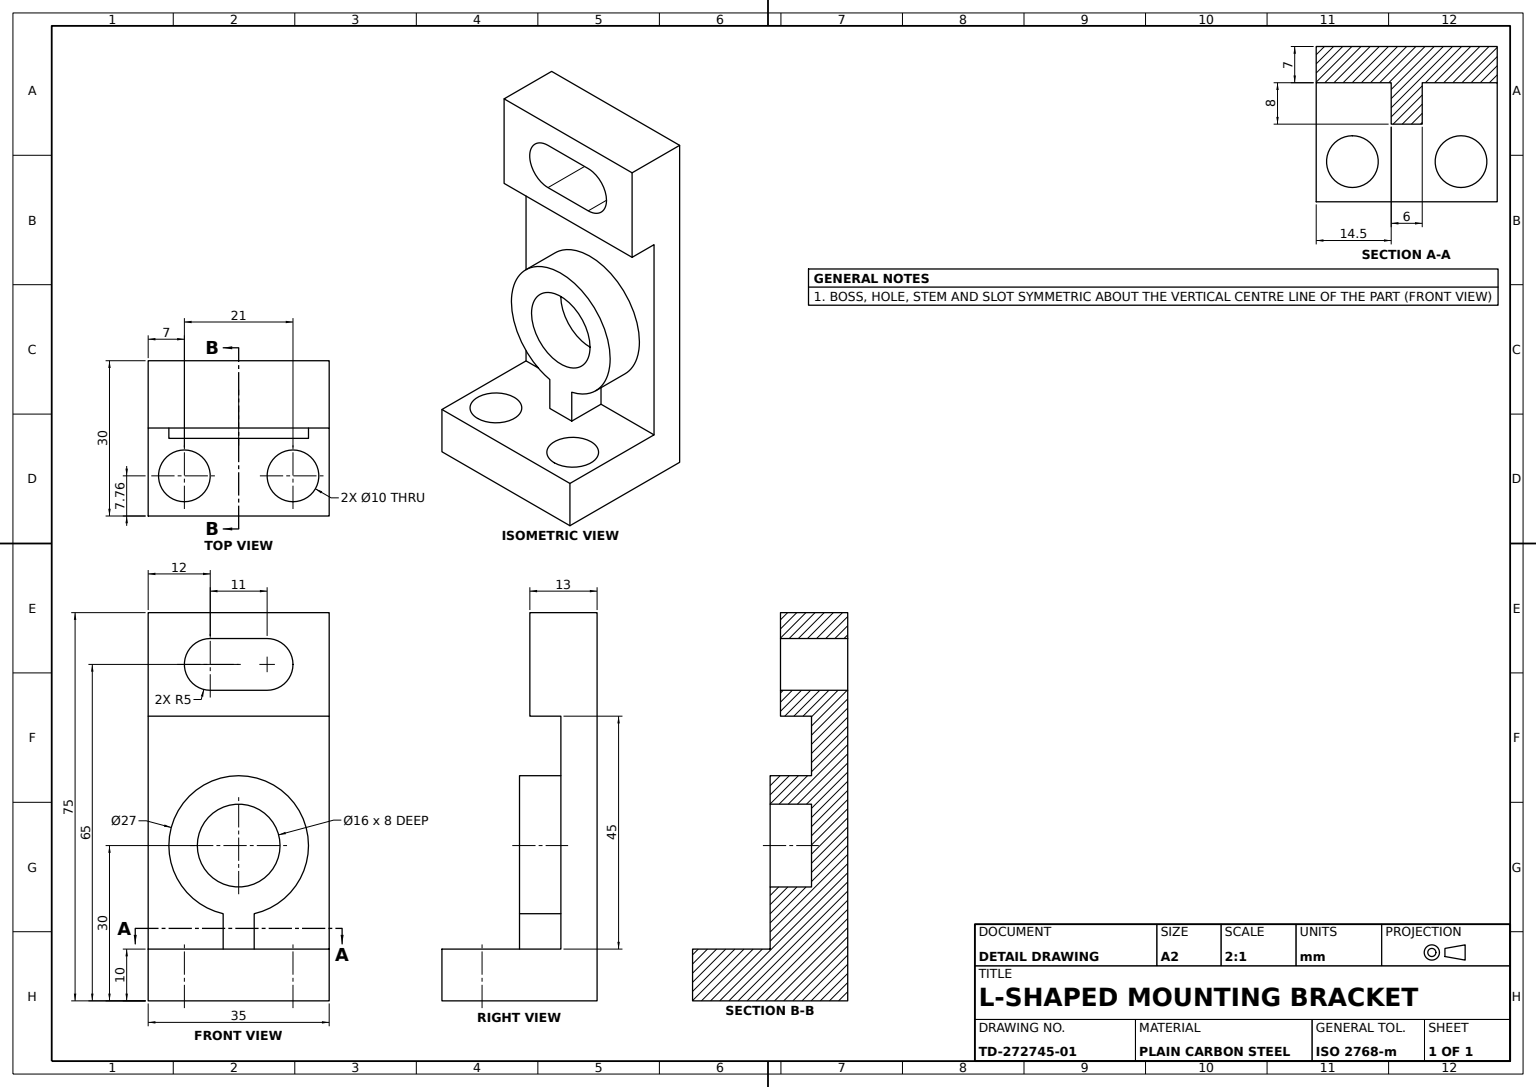
SolidWorks part; units mm, degrees
material "Plain Carbon Steel"
ref_plane "Front Plane" through (0, 0, 0) normal (0, 0, 1) x (1, 0, 0)
ref_plane "Top Plane" through (0, 0, 0) normal (0, 1, 0) x (1, 0, 0)
ref_plane "Right Plane" through (0, 0, 0) normal (1, 0, 0) x (0, 0, -1)
sketch "L-Bracket Profile Sketch" plane through (0, 0, 0) normal (1, 0, 0) x (0, 0, -1)
  line L0 (0, 0) -> (30, 0)
  line L1 (30, 0) -> (30, 10)
  line L2 (30, 10) -> (7, 10)
  line L3 (7, 10) -> (7, 55)
  line L4 (7, 55) -> (13, 55)
  line L5 (13, 55) -> (13, 75)
  line L6 (13, 75) -> (0, 75)
  line L7 (0, 75) -> (0, 0)
  dimension "D1" = 30
  dimension "D2" = 75
  dimension "D3" = 20
  dimension "D4" = 45
  dimension "D5" = 13
  dimension "D6" = 6
extrude "L-Bracket Body" add sketch "L-Bracket Profile Sketch" along normal mid plane 35
sketch "Upright Slot Sketch" plane through (0, 0, -13) normal (0, 0, -1) x (-1, 0, 0)
  line L0 (-5.5, 65) -> (5.5, 65) construction
  line L1 (-5.5, 70) -> (5.5, 70)
  line L2 (-5.5, 60) -> (5.5, 60)
  arc A0 (-5.5, 70) -> (-5.5, 60) centre (-5.5, 65) ccw
  arc A1 (5.5, 60) -> (5.5, 70) centre (5.5, 65) ccw
  point P2 (0, 65)
  dimension "D1" = 5
  dimension "D2" = 11
  dimension "D3" = 65
extrude "Upright Slot" cut sketch "Upright Slot Sketch" against normal blind 35
sketch "Corner Support Boss Sketch" plane through (0, 0, -7) normal (0, 0, -1) x (-1, 0, 0)
  line L0 (-17.5, 10) -> (17.5, 10) construction
  line L1 (-3, 16.8376) -> (-3, 10)
  line L2 (3, 16.8376) -> (3, 10)
  line L3 (-3, 10) -> (3, 10)
  arc A0 (3, 16.8376) -> (-3, 16.8376) centre (0, 30) ccw
  circle A1 centre (0, 30) radius 8
  dimension "D1" = 16
  dimension "D2" = 27
  dimension "D3" = 30
  dimension "D4" = 6
  dimension "D5" = 3
extrude "Corner Support Boss" add sketch "Corner Support Boss Sketch" along normal blind 8
hole_wizard "Dowel Hole Ø10" positions "Sketch4" profile "Sketch5" hole size "Ø1.0" standard "ANSI Metric" end condition through all
sketch "Sketch4" plane through (0, 10, 0) normal (0, 1, 0) x (1, 0, 0)
  point P0 (-10.5, 22.2406)
  point P2 (10.5, 22.2406)
  dimension "D1" = 21
  dimension "D2" = 10.5
sketch "Sketch5" plane through (-10.5, 10, -22.2406) normal (1, 0, 0) x (0, 0, 1)
  line L0 (0, 0) -> (0, 10)
  line L1 (0, 10) -> (5, 10)
  line L2 (5, 10) -> (5, 0)
  line L5 (5, 0) -> (0, 0)
  line L11 (0, -6.35) -> (0, 107.95) construction
  dimension "Thru Hole Dia." = 10
  dimension "Thru Hole Depth" = 10
